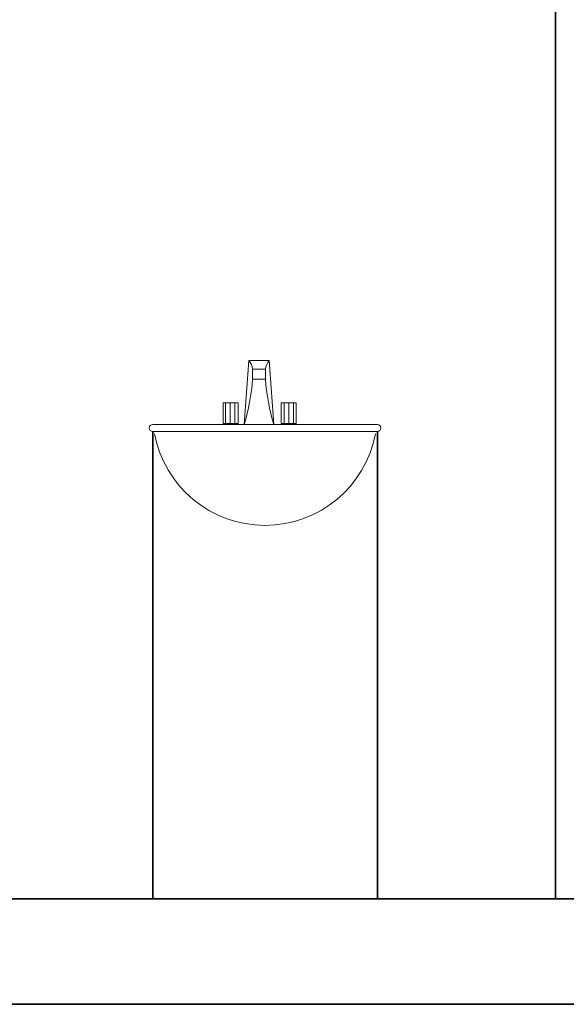
# Model space of a CAD drawing. Units: inches. Extents: x 64 to 1167, y 117 to 939.
# Tile 37 of 56: x 1074 to 1121, y 428 to 512. Entities that reach past the tile are written whole.
import ezdxf

# ---------------------------------------------------------------- set-up
doc = ezdxf.new("R2010")
doc.units = ezdxf.units.IN
doc.header["$MEASUREMENT"] = 0
doc.layers.add('A-FLOR-FIXT', color=8, linetype='Continuous', lineweight=18)
doc.layers.add('A-SECT', color=7, linetype='Continuous', lineweight=35)

# ---------------------------------------------------------------- blocks, each defined once
blk = doc.blocks.new('A$C52D46D27')
for p, q in [((0.2156, 0.3476), (0.2056, 0.2089)), ((0.2597, 0.3476), (0.2156, 0.3476)), ((0.2697, 0.2089), (0.2597, 0.3476)), ((0.2236, 0.3288), (0.2236, 0.3075)), ((0.2516, 0.3288), (0.2236, 0.3288)), ((0.2516, 0.3288), (0.2516, 0.3075)), ((0.2236, 0.3075), (0.2516, 0.3075)), ((0.1601, 0.2559), (0.1601, 0.2112)), ((0.1922, 0.2559), (0.1601, 0.2559)), ((0.1652, 0.2559), (0.1652, 0.2112)), ((0.1752, 0.2559), (0.1752, 0.2112)), ((0.1852, 0.2559), (0.1852, 0.2112)), ((0.1922, 0.2112), (0.1922, 0.2559)), ((0.2858, 0.2112), (0.2858, 0.2559)), ((0.2858, 0.2559), (0.3179, 0.2559)), ((0.2923, 0.2559), (0.2923, 0.2112)), ((0.3023, 0.2559), (0.3023, 0.2112)), ((0.3123, 0.2559), (0.3123, 0.2112)), ((0.3179, 0.2559), (0.3179, 0.2112)), ((0.4938, 0.2091), (0.0075, 0.2091)), ((0.4938, 0.1941), (0.0075, 0.1941)), ((0.1601, 0.2112), (0.1922, 0.2112)), ((0.2056, 0.2089), (0.2697, 0.2089)), ((0.3179, 0.2112), (0.2858, 0.2112))]:
    blk.add_line(p, q)
for centre, radius, start, end in [((0.1895, 0.3254), 0.0343, 5.6725, 40.4808), ((0.2858, 0.3254), 0.0343, 139.5192, 174.3275), ((-0.2336, 0.3401), 0.4584, 343.3578, 355.9235), ((0.7088, 0.3401), 0.4584, 184.0765, 196.6422), ((0.0075, 0.2016), 0.0075, 90, 270), ((0.4938, 0.2016), 0.0075, 270, 90)]:
    blk.add_arc(centre, radius, start, end)
at = {"ltscale": 10}
blk.add_arc((0.2505, 0.2339), 0.2432, 190.628, 349.372, dxfattribs=at)

msp = doc.modelspace()

# ---------------------------------------------------------------- linework, layer by layer
at = {"layer": 'A-SECT'}
for p, q in [((1119.813, 436.679), (1119.813, 540.679)), ((1085.492, 476.505), (1085.492, 436.679)), ((1104.636, 476.505), (1104.636, 436.679)), ((991.813, 436.679), (1157.813, 436.679))]:
    msp.add_line(p, q, dxfattribs=at)
msp.add_lwpolyline([(982.813, 427.679), (1166.813, 427.679), (1166.813, 565.679), (982.813, 565.679)], close=True, dxfattribs=at)

# ---------------------------------------------------------------- block references
at = {"layer": 'A-FLOR-FIXT', "xscale": 39.37007874015748, "yscale": 39.37007874015748, "zscale": 39.37007874015748}
msp.add_blockref('A$C52D46D27', (1085.197, 468.865), dxfattribs=at)

doc.saveas('drawing.dxf')
